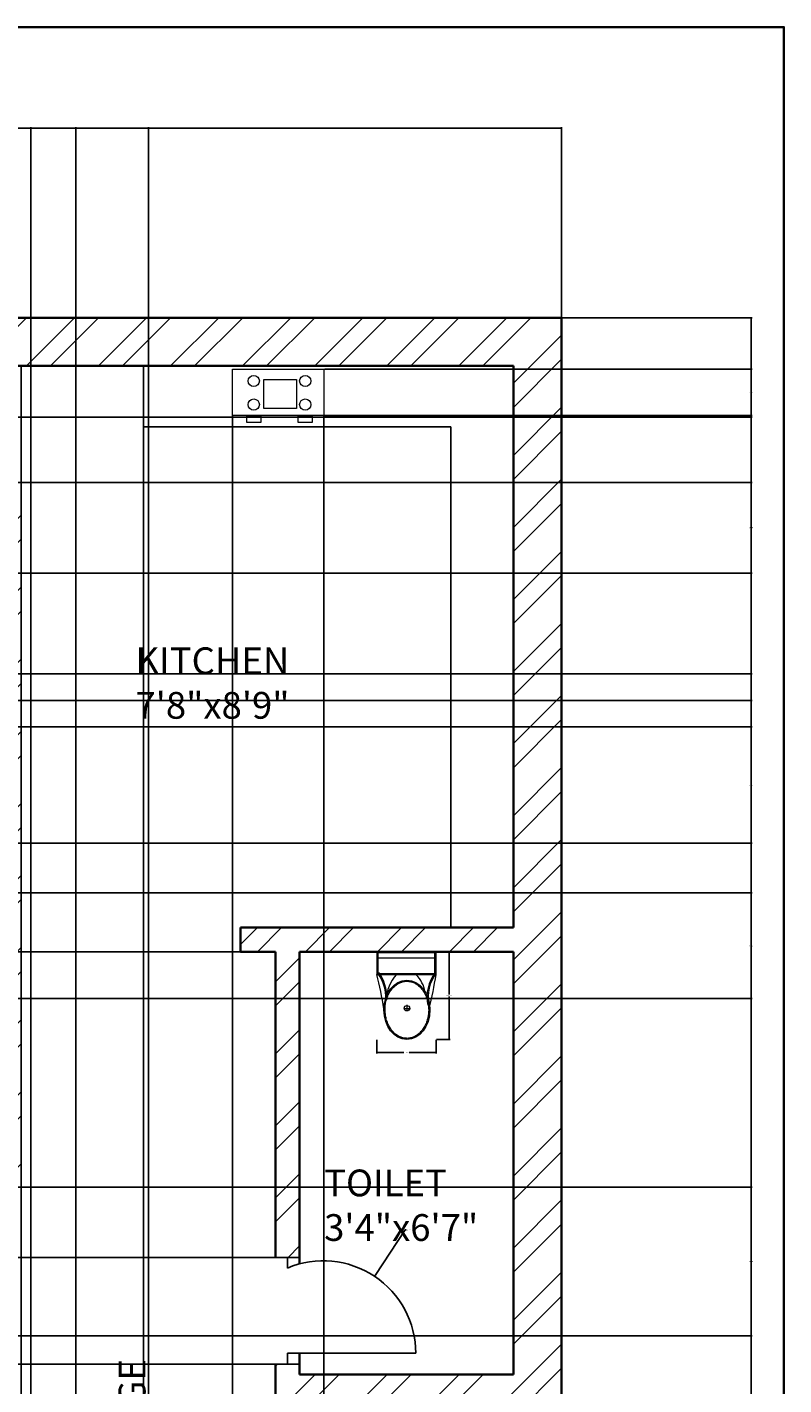
# Model space of a CAD drawing. Units: inches. Extents: x 2529 to 3014, y 1203 to 2262.
# Tile 13 of 13: x 2872 to 3014, y 2008 to 2262. Entities that reach past the tile are written whole.
import ezdxf

# ---------------------------------------------------------------- set-up
doc = ezdxf.new("R2010")
doc.units = ezdxf.units.IN
for name, color, linetype, lineweight in [('A-ANNO-DIMS', 2, 'Continuous', 18), ('A-ANNO-TTLB', 7, 'Continuous', 35), ('A-AREA-IDEN', 7, 'Continuous', 18), ('A-DOOR', 21, 'Continuous', 25), ('A-EQPM', 8, 'Continuous', 18), ('A-FLOR-CASE', 7, 'Continuous', 25), ('A-FLOR-FIXT', 8, 'Continuous', 18), ('A-WALL', 7, 'Continuous', 35), ('A-WALL-PATT', 143, 'Continuous', 13)]:
    doc.layers.add(name, color=color, linetype=linetype, lineweight=lineweight)
doc.styles.get("Standard").update_dxf_attribs({"font": 'arial.ttf'})
doc.dimstyles.get("Standard").update_dxf_attribs({"dimtxt": 0.18, "dimasz": 0.18, "dimexe": 0.18, "dimexo": 0.0625, "dimgap": 0.09, "dimtad": 0, "dimtih": 1, "dimtoh": 1, "dimdec": 4, "dimzin": 0, "dimdsep": 46, "dimtxsty": 'Standard', "dimcen": 0.09, "dimadec": 0, "dimazin": 0, "dimtfac": 1, "dimtdec": 4, "dimtofl": 0, "dimtmove": 0, "dimatfit": 3, "dimfxl": 1, "dimtolj": 1, "dimtzin": 0, "dimarcsym": 0})

# ---------------------------------------------------------------- blocks, each defined once
blk = doc.blocks.new('A$C31115884')
for p, q in [((283, 498), (223, 498)), ((258, 466), (258, 523)), ((0, 200), (0, 0)), ((520, 200), (0, 200)), ((10, 190), (10, 10)), ((510, 190), (10, 190)), ((510, 10), (510, 190)), ((520, 0), (520, 200)), ((510, 54), (0, 54)), ((10, 10), (510, 10)), ((0, 0), (520, 0))]:
    blk.add_line(p, q)
blk.add_circle((256, 496), 23.6)
for centre, radius, start, end in [((2778, -205), 2807, 165.4549, 171.7133), ((3237, 905), 2807, 188.2867, 194.5451), ((-295, 403), 365, 324.2091, 9.3499), ((-295, 403), 375, 324.2091, 9.3499), ((139, 406), 293, 315.8436, 2.6563), ((806, 403), 375, 179.2036, 215.7909), ((806, 403), 365, 170.6501, 215.7909), ((384, 406), 293, 190.2774, 224.1564)]:
    blk.add_arc(centre, radius, start, end)
blk.add_ellipse((256, 510), major_axis=(0, -261), ratio=0.772727)
blk.add_open_spline([(256, 259), (263, 259), (270, 260), (288, 262), (299, 265), (320, 273), (330, 278), (350, 291), (360, 299), (378, 316), (386, 326), (402, 347), (409, 358), (421, 383), (427, 395), (436, 422), (440, 436), (445, 465), (447, 480), (448, 509), (448, 524), (445, 553), (443, 568), (436, 596), (432, 610), (422, 636), (416, 649), (402, 672), (395, 683), (379, 703), (370, 712), (351, 728), (341, 735), (321, 746), (310, 751), (289, 757), (278, 759), (256, 761), (245, 761), (223, 757), (212, 754), (191, 746), (181, 741), (161, 728), (151, 720), (133, 703), (125, 693), (110, 672), (103, 660), (90, 636), (85, 623), (76, 596), (72, 582), (67, 553), (66, 538), (64, 509), (65, 494), (68, 465), (70, 450), (77, 422), (81, 408), (91, 382), (97, 370), (111, 346), (118, 335), (135, 316), (144, 307), (162, 291), (172, 284), (193, 273), (203, 269), (225, 262), (236, 260), (250, 259), (253, 259), (256, 259)], degree=3, knots=[0, 0, 0, 0, 0.110105, 0.110105, 0.285049, 0.285049, 0.459994, 0.459994, 0.634938, 0.634938, 0.809882, 0.809882, 0.984827, 0.984827, 1.159771, 1.159771, 1.334715, 1.334715, 1.50966, 1.50966, 1.684604, 1.684604, 1.859549, 1.859549, 2.034493, 2.034493, 2.209437, 2.209437, 2.384382, 2.384382, 2.559326, 2.559326, 2.73427, 2.73427, 2.909215, 2.909215, 3.084159, 3.084159, 3.259103, 3.259103, 3.434048, 3.434048, 3.608992, 3.608992, 3.783936, 3.783936, 3.958881, 3.958881, 4.133825, 4.133825, 4.30877, 4.30877, 4.483714, 4.483714, 4.658658, 4.658658, 4.833603, 4.833603, 5.008547, 5.008547, 5.183491, 5.183491, 5.358436, 5.358436, 5.53338, 5.53338, 5.708324, 5.708324, 5.883269, 5.883269, 6.058213, 6.058213, 6.233158, 6.233158, 6.283185, 6.283185, 6.283185, 6.283185])
blk = doc.blocks.new('*D8')
at = {"layer": 'A-ANNO-DIMS', "color": 0, "lineweight": -2, "transparency": 16777216}
for p, q in [((2948.65, 2089), (2951.23, 2089)), ((2951.05, 2088.82), (2951.05, 2080.99)), ((2951.05, 2072.78), (2951.05, 2080.62)), ((2948.65, 2072.6), (2951.23, 2072.6))]:
    blk.add_line(p, q, dxfattribs=at)
at = {"layer": 'A-ANNO-DIMS', "color": 0, "transparency": 16777216}
for points in [[(2951.02, 2088.82), (2951.08, 2088.82), (2951.05, 2089)], [(2951.02, 2072.78), (2951.08, 2072.78), (2951.05, 2072.6)]]:
    blk.add_solid(points, dxfattribs=at)
at = {"layer": 'Defpoints', "color": 0, "transparency": 16777216}
for p in [(2948.59, 2089), (2948.59, 2072.6), (2951.05, 2072.6)]:
    blk.add_point(p, dxfattribs=at)
at = {"layer": 'A-ANNO-DIMS', "color": 0, "transparency": 16777216, "insert": (2951.05, 2080.8), "char_height": 0.18, "attachment_point": 5}
blk.add_mtext('\\A1;WC 16 TYP.', dxfattribs=at)
blk = doc.blocks.new('*D9')
at = {"layer": 'A-ANNO-DIMS', "color": 0, "lineweight": -2, "transparency": 16777216}
for p, q in [((2937.52, 2072.54), (2937.52, 2069.96)), ((2948.59, 2072.54), (2948.59, 2069.96)), ((2937.7, 2070.14), (2942.54, 2070.14)), ((2948.41, 2070.14), (2943.57, 2070.14))]:
    blk.add_line(p, q, dxfattribs=at)
at = {"layer": 'A-ANNO-DIMS', "color": 0, "transparency": 16777216}
for points in [[(2937.7, 2070.17), (2937.7, 2070.11), (2937.52, 2070.14)], [(2948.41, 2070.17), (2948.41, 2070.11), (2948.59, 2070.14)]]:
    blk.add_solid(points, dxfattribs=at)
at = {"layer": 'Defpoints', "color": 0, "transparency": 16777216}
for p in [(2937.52, 2072.6), (2948.59, 2072.6), (2937.52, 2070.14)]:
    blk.add_point(p, dxfattribs=at)
at = {"layer": 'A-ANNO-DIMS', "color": 0, "transparency": 16777216, "insert": (2943.06, 2070.14), "char_height": 0.18, "attachment_point": 5}
blk.add_mtext('\\A1;11 TYP.', dxfattribs=at)
blk = doc.blocks.new('*D16')
at = {"layer": 'A-ANNO-DIMS', "color": 0, "lineweight": -2, "transparency": 16777216}
for p, q in [((2577.06, 2207.57), (2577.06, 2243.11)), ((2577.24, 2242.93), (2774.27, 2242.93)), ((2971.88, 2242.93), (2774.84, 2242.93)), ((2972.06, 2207.57), (2972.06, 2243.11))]:
    blk.add_line(p, q, dxfattribs=at)
at = {"layer": 'A-ANNO-DIMS', "color": 0, "transparency": 16777216}
for points in [[(2577.24, 2242.96), (2577.24, 2242.9), (2577.06, 2242.93)], [(2971.88, 2242.96), (2971.88, 2242.9), (2972.06, 2242.93)]]:
    blk.add_solid(points, dxfattribs=at)
at = {"layer": 'Defpoints', "color": 0, "transparency": 16777216}
for p in [(2972.06, 2242.93), (2577.06, 2207.5), (2972.06, 2207.5)]:
    blk.add_point(p, dxfattribs=at)
at = {"layer": 'A-ANNO-DIMS', "color": 0, "transparency": 16777216, "insert": (2774.56, 2242.93), "char_height": 0.18, "attachment_point": 5}
blk.add_mtext('\\A1;395', dxfattribs=at)
blk = doc.blocks.new('*D17')
at = {"layer": 'A-ANNO-DIMS', "color": 0, "lineweight": -2, "transparency": 16777216}
for p, q in [((2972.12, 2207.5), (3007.66, 2207.5)), ((3007.48, 2207.32), (3007.48, 1890.69)), ((3007.48, 1573.68), (3007.48, 1890.32)), ((2972.12, 1573.5), (3007.66, 1573.5))]:
    blk.add_line(p, q, dxfattribs=at)
at = {"layer": 'A-ANNO-DIMS', "color": 0, "transparency": 16777216}
for points in [[(3007.45, 2207.32), (3007.51, 2207.32), (3007.48, 2207.5)], [(3007.45, 1573.68), (3007.51, 1573.68), (3007.48, 1573.5)]]:
    blk.add_solid(points, dxfattribs=at)
at = {"layer": 'Defpoints', "color": 0, "transparency": 16777216}
for p in [(2972.06, 2207.5), (3007.48, 2207.5), (2972.06, 1573.5)]:
    blk.add_point(p, dxfattribs=at)
at = {"layer": 'A-ANNO-DIMS', "color": 0, "transparency": 16777216, "insert": (3007.48, 1890.5), "char_height": 0.18, "attachment_point": 5}
blk.add_mtext('\\A1;634', dxfattribs=at)
blk = doc.blocks.new('*D39')
at = {"layer": 'A-ANNO-DIMS', "color": 0, "lineweight": -2, "transparency": 16777216}
for p, q in [((2848.27, 1734.07), (2848.27, 2243.11)), ((2848.45, 2242.93), (2864.3, 2242.93)), ((2881.08, 2242.93), (2865.23, 2242.93)), ((2881.26, 1734.07), (2881.26, 2243.11))]:
    blk.add_line(p, q, dxfattribs=at)
at = {"layer": 'A-ANNO-DIMS', "color": 0, "transparency": 16777216}
for points in [[(2848.45, 2242.96), (2848.45, 2242.9), (2848.27, 2242.93)], [(2881.08, 2242.96), (2881.08, 2242.9), (2881.26, 2242.93)]]:
    blk.add_solid(points, dxfattribs=at)
at = {"layer": 'Defpoints', "color": 0, "transparency": 16777216}
for p in [(2881.26, 2242.93), (2848.27, 1734), (2881.26, 1734)]:
    blk.add_point(p, dxfattribs=at)
at = {"layer": 'A-ANNO-DIMS', "color": 0, "transparency": 16777216, "insert": (2864.76, 2242.93), "char_height": 0.18, "attachment_point": 5}
blk.add_mtext('\\A1;32.994', dxfattribs=at)
blk = doc.blocks.new('*D46')
at = {"layer": 'A-ANNO-DIMS', "color": 0, "lineweight": -2, "transparency": 16777216}
for p, q in [((2613.12, 2188.94), (3007.66, 2188.94)), ((3007.48, 2188.76), (3007.48, 2165.12)), ((3007.48, 2141.12), (3007.48, 2164.75)), ((2613.12, 2140.94), (3007.66, 2140.94))]:
    blk.add_line(p, q, dxfattribs=at)
at = {"layer": 'A-ANNO-DIMS', "color": 0, "transparency": 16777216}
for points in [[(3007.45, 2188.76), (3007.51, 2188.76), (3007.48, 2188.94)], [(3007.45, 2141.12), (3007.51, 2141.12), (3007.48, 2140.94)]]:
    blk.add_solid(points, dxfattribs=at)
at = {"layer": 'Defpoints', "color": 0, "transparency": 16777216}
for p in [(2613.06, 2188.94), (3007.48, 2188.94), (2613.06, 2140.94)]:
    blk.add_point(p, dxfattribs=at)
at = {"layer": 'A-ANNO-DIMS', "color": 0, "transparency": 16777216, "insert": (3007.48, 2164.94), "char_height": 0.18, "attachment_point": 5}
blk.add_mtext('\\A1;48', dxfattribs=at)
blk = doc.blocks.new('*D47')
at = {"layer": 'A-ANNO-DIMS', "color": 0, "lineweight": -2, "transparency": 16777216}
for p, q in [((2622.12, 2131.02), (3007.66, 2131.02)), ((3007.48, 2130.84), (3007.48, 2120.34)), ((3007.48, 2109.48), (3007.48, 2119.98)), ((2622.12, 2109.3), (3007.66, 2109.3))]:
    blk.add_line(p, q, dxfattribs=at)
at = {"layer": 'A-ANNO-DIMS', "color": 0, "transparency": 16777216}
for points in [[(3007.45, 2130.84), (3007.51, 2130.84), (3007.48, 2131.02)], [(3007.45, 2109.48), (3007.51, 2109.48), (3007.48, 2109.3)]]:
    blk.add_solid(points, dxfattribs=at)
at = {"layer": 'Defpoints', "color": 0, "transparency": 16777216}
for p in [(2622.06, 2131.02), (3007.48, 2131.02), (2622.06, 2109.3)]:
    blk.add_point(p, dxfattribs=at)
at = {"layer": 'A-ANNO-DIMS', "color": 0, "transparency": 16777216, "insert": (3007.48, 2120.16), "char_height": 0.18, "attachment_point": 5}
blk.add_mtext('\\A1;21.72', dxfattribs=at)
blk = doc.blocks.new('*D48')
at = {"layer": 'A-ANNO-DIMS', "color": 0, "lineweight": -2, "transparency": 16777216}
for p, q in [((2686.62, 2099.98), (3007.66, 2099.98)), ((3007.48, 2099.8), (3007.48, 2090.29)), ((3007.48, 2080.41), (3007.48, 2089.93)), ((2686.62, 2080.23), (3007.66, 2080.23))]:
    blk.add_line(p, q, dxfattribs=at)
at = {"layer": 'A-ANNO-DIMS', "color": 0, "transparency": 16777216}
for points in [[(3007.45, 2099.8), (3007.51, 2099.8), (3007.48, 2099.98)], [(3007.45, 2080.41), (3007.51, 2080.41), (3007.48, 2080.23)]]:
    blk.add_solid(points, dxfattribs=at)
at = {"layer": 'Defpoints', "color": 0, "transparency": 16777216}
for p in [(2686.56, 2099.98), (3007.48, 2099.98), (2686.56, 2080.23)]:
    blk.add_point(p, dxfattribs=at)
at = {"layer": 'A-ANNO-DIMS', "color": 0, "transparency": 16777216, "insert": (3007.48, 2090.11), "char_height": 0.18, "attachment_point": 5}
blk.add_mtext('\\A1;19.75', dxfattribs=at)
blk = doc.blocks.new('*D50')
at = {"layer": 'A-ANNO-DIMS', "color": 0, "lineweight": -2, "transparency": 16777216}
for p, q in [((2866.62, 2045.02), (3007.66, 2045.02)), ((3007.48, 2044.84), (3007.48, 2031.3)), ((3007.48, 2017.39), (3007.48, 2030.93)), ((2866.62, 2017.21), (3007.66, 2017.21))]:
    blk.add_line(p, q, dxfattribs=at)
at = {"layer": 'A-ANNO-DIMS', "color": 0, "transparency": 16777216}
for points in [[(3007.45, 2044.84), (3007.51, 2044.84), (3007.48, 2045.02)], [(3007.45, 2017.39), (3007.51, 2017.39), (3007.48, 2017.21)]]:
    blk.add_solid(points, dxfattribs=at)
at = {"layer": 'Defpoints', "color": 0, "transparency": 16777216}
for p in [(2866.56, 2045.02), (3007.48, 2045.02), (2866.56, 2017.21)]:
    blk.add_point(p, dxfattribs=at)
at = {"layer": 'A-ANNO-DIMS', "color": 0, "transparency": 16777216, "insert": (3007.48, 2031.12), "char_height": 0.18, "attachment_point": 5}
blk.add_mtext('\\A1;27.814', dxfattribs=at)
blk = doc.blocks.new('*D57')
at = {"layer": 'A-ANNO-DIMS', "color": 0, "lineweight": -2, "transparency": 16777216}
for p, q in [((2871.06, 2198.44), (2871.06, 1483.77)), ((2893.92, 2198.44), (2893.92, 1483.77)), ((2871.24, 1483.95), (2882.02, 1483.95)), ((2893.74, 1483.95), (2882.95, 1483.95))]:
    blk.add_line(p, q, dxfattribs=at)
at = {"layer": 'A-ANNO-DIMS', "color": 0, "transparency": 16777216}
for points in [[(2871.24, 1483.98), (2871.24, 1483.92), (2871.06, 1483.95)], [(2893.74, 1483.98), (2893.74, 1483.92), (2893.92, 1483.95)]]:
    blk.add_solid(points, dxfattribs=at)
at = {"layer": 'Defpoints', "color": 0, "transparency": 16777216}
for p in [(2871.06, 2198.5), (2893.92, 2198.5), (2893.92, 1483.95)]:
    blk.add_point(p, dxfattribs=at)
at = {"layer": 'A-ANNO-DIMS', "color": 0, "transparency": 16777216, "insert": (2882.49, 1483.95), "char_height": 0.18, "attachment_point": 5}
blk.add_mtext('\\A1;22.866', dxfattribs=at)
blk = doc.blocks.new('*D58')
at = {"layer": 'A-ANNO-DIMS', "color": 0, "lineweight": -2, "transparency": 16777216}
for p, q in [((2918.49, 2089), (2541.45, 2089)), ((2541.63, 2088.82), (2541.63, 2060.62)), ((2541.63, 2032.05), (2541.63, 2060.26)), ((2918.49, 2031.87), (2541.45, 2031.87))]:
    blk.add_line(p, q, dxfattribs=at)
at = {"layer": 'A-ANNO-DIMS', "color": 0, "transparency": 16777216}
for points in [[(2541.6, 2088.82), (2541.66, 2088.82), (2541.63, 2089)], [(2541.6, 2032.05), (2541.66, 2032.05), (2541.63, 2031.87)]]:
    blk.add_solid(points, dxfattribs=at)
at = {"layer": 'Defpoints', "color": 0, "transparency": 16777216}
for p in [(2918.56, 2089), (2541.63, 2031.87), (2918.56, 2031.87)]:
    blk.add_point(p, dxfattribs=at)
at = {"layer": 'A-ANNO-DIMS', "color": 0, "transparency": 16777216, "insert": (2541.63, 2060.44), "char_height": 0.18, "attachment_point": 5}
blk.add_mtext('\\A1;57.13', dxfattribs=at)
blk = doc.blocks.new('*D59')
at = {"layer": 'A-ANNO-DIMS', "color": 0, "lineweight": -2, "transparency": 16777216}
for p, q in [((2918.49, 2031.87), (2541.45, 2031.87)), ((2541.63, 2031.69), (2541.63, 2022.09)), ((2541.63, 2012.12), (2541.63, 2021.73)), ((2918.49, 2011.94), (2541.45, 2011.94))]:
    blk.add_line(p, q, dxfattribs=at)
at = {"layer": 'A-ANNO-DIMS', "color": 0, "transparency": 16777216}
for points in [[(2541.6, 2031.69), (2541.66, 2031.69), (2541.63, 2031.87)], [(2541.6, 2012.12), (2541.66, 2012.12), (2541.63, 2011.94)]]:
    blk.add_solid(points, dxfattribs=at)
at = {"layer": 'Defpoints', "color": 0, "transparency": 16777216}
for p in [(2918.56, 2031.87), (2541.63, 2011.94), (2918.56, 2011.94)]:
    blk.add_point(p, dxfattribs=at)
at = {"layer": 'A-ANNO-DIMS', "color": 0, "transparency": 16777216, "insert": (2541.63, 2021.91), "char_height": 0.18, "attachment_point": 5}
blk.add_mtext('\\A1;19.933', dxfattribs=at)
blk = doc.blocks.new('*D64')
at = {"layer": 'A-ANNO-DIMS', "color": 0, "lineweight": -2, "transparency": 16777216}
for p, q in [((2872.87, 1791.07), (2872.87, 2243.11)), ((2873.05, 2242.93), (2883.47, 2242.93)), ((2894.68, 2242.93), (2884.26, 2242.93)), ((2894.86, 1791.07), (2894.86, 2243.11))]:
    blk.add_line(p, q, dxfattribs=at)
at = {"layer": 'A-ANNO-DIMS', "color": 0, "transparency": 16777216}
for points in [[(2873.05, 2242.96), (2873.05, 2242.9), (2872.87, 2242.93)], [(2894.68, 2242.96), (2894.68, 2242.9), (2894.86, 2242.93)]]:
    blk.add_solid(points, dxfattribs=at)
at = {"layer": 'Defpoints', "color": 0, "transparency": 16777216}
for p in [(2894.86, 2242.93), (2872.87, 1791), (2894.86, 1791)]:
    blk.add_point(p, dxfattribs=at)
at = {"layer": 'A-ANNO-DIMS', "color": 0, "transparency": 16777216, "insert": (2883.87, 2242.93), "char_height": 0.18, "attachment_point": 5}
blk.add_mtext('\\A1;21.99', dxfattribs=at)
blk = doc.blocks.new('*D72')
at = {"layer": 'A-ANNO-DIMS', "color": 0, "lineweight": -2, "transparency": 16777216}
for p, q in [((2631.64, 2176.7), (3007.66, 2176.7)), ((3007.48, 2176.52), (3007.48, 2168.41)), ((3007.48, 2159.93), (3007.48, 2168.04)), ((2631.64, 2159.75), (3007.66, 2159.75))]:
    blk.add_line(p, q, dxfattribs=at)
at = {"layer": 'A-ANNO-DIMS', "color": 0, "transparency": 16777216}
for points in [[(3007.45, 2176.52), (3007.51, 2176.52), (3007.48, 2176.7)], [(3007.45, 2159.93), (3007.51, 2159.93), (3007.48, 2159.75)]]:
    blk.add_solid(points, dxfattribs=at)
at = {"layer": 'Defpoints', "color": 0, "transparency": 16777216}
for p in [(2631.58, 2176.7), (3007.48, 2176.7), (2631.58, 2159.75)]:
    blk.add_point(p, dxfattribs=at)
at = {"layer": 'A-ANNO-DIMS', "color": 0, "transparency": 16777216, "insert": (3007.48, 2168.22), "char_height": 0.18, "attachment_point": 5}
blk.add_mtext('\\A1;16.957', dxfattribs=at)
blk = doc.blocks.new('*D73')
at = {"layer": 'A-ANNO-DIMS', "color": 0, "lineweight": -2, "transparency": 16777216}
for p, q in [((2631.64, 2159.75), (3007.66, 2159.75)), ((3007.48, 2159.57), (3007.48, 2148.04)), ((3007.48, 2136.16), (3007.48, 2147.68)), ((2634.12, 2135.98), (3007.66, 2135.98))]:
    blk.add_line(p, q, dxfattribs=at)
at = {"layer": 'A-ANNO-DIMS', "color": 0, "transparency": 16777216}
for points in [[(3007.45, 2159.57), (3007.51, 2159.57), (3007.48, 2159.75)], [(3007.45, 2136.16), (3007.51, 2136.16), (3007.48, 2135.98)]]:
    blk.add_solid(points, dxfattribs=at)
at = {"layer": 'Defpoints', "color": 0, "transparency": 16777216}
for p in [(2631.58, 2159.75), (2634.06, 2135.98), (3007.48, 2135.98)]:
    blk.add_point(p, dxfattribs=at)
at = {"layer": 'A-ANNO-DIMS', "color": 0, "transparency": 16777216, "insert": (3007.48, 2147.86), "char_height": 0.18, "attachment_point": 5}
blk.add_mtext('\\A1;23.77', dxfattribs=at)
blk = doc.blocks.new('*D75')
at = {"layer": 'A-ANNO-DIMS', "color": 0, "lineweight": -2, "transparency": 16777216}
for p, q in [((2910.52, 2189.17), (2910.52, 1483.77)), ((2893.92, 2187.06), (2893.92, 1483.77)), ((2894.1, 1483.95), (2901.91, 1483.95)), ((2910.34, 1483.95), (2902.54, 1483.95))]:
    blk.add_line(p, q, dxfattribs=at)
at = {"layer": 'A-ANNO-DIMS', "color": 0, "transparency": 16777216}
for points in [[(2894.1, 1483.98), (2894.1, 1483.92), (2893.92, 1483.95)], [(2910.34, 1483.98), (2910.34, 1483.92), (2910.52, 1483.95)]]:
    blk.add_solid(points, dxfattribs=at)
at = {"layer": 'Defpoints', "color": 0, "transparency": 16777216}
for p in [(2910.52, 2189.24), (2893.92, 2187.12), (2910.52, 1483.95)]:
    blk.add_point(p, dxfattribs=at)
at = {"layer": 'A-ANNO-DIMS', "color": 0, "transparency": 16777216, "insert": (2902.22, 1483.95), "char_height": 0.18, "attachment_point": 5}
blk.add_mtext('\\A1;16.6', dxfattribs=at)
blk = doc.blocks.new('*D76')
at = {"layer": 'A-ANNO-DIMS', "color": 0, "lineweight": -2, "transparency": 16777216}
for p, q in [((2910.52, 2189.17), (2910.52, 1483.77)), ((2927.64, 2189.17), (2927.64, 1483.77)), ((2910.7, 1483.95), (2918.63, 1483.95)), ((2927.46, 1483.95), (2919.54, 1483.95))]:
    blk.add_line(p, q, dxfattribs=at)
at = {"layer": 'A-ANNO-DIMS', "color": 0, "transparency": 16777216}
for points in [[(2910.7, 1483.98), (2910.7, 1483.92), (2910.52, 1483.95)], [(2927.46, 1483.98), (2927.46, 1483.92), (2927.64, 1483.95)]]:
    blk.add_solid(points, dxfattribs=at)
at = {"layer": 'Defpoints', "color": 0, "transparency": 16777216}
for p in [(2910.52, 2189.24), (2927.64, 2189.24), (2927.64, 1483.95)]:
    blk.add_point(p, dxfattribs=at)
at = {"layer": 'A-ANNO-DIMS', "color": 0, "transparency": 16777216, "insert": (2919.08, 1483.95), "char_height": 0.18, "attachment_point": 5}
blk.add_mtext('\\A1;17.123', dxfattribs=at)
blk = doc.blocks.new('*D77')
at = {"layer": 'A-ANNO-DIMS', "color": 0, "lineweight": -2, "transparency": 16777216}
for p, q in [((2927.71, 2197.87), (3007.66, 2197.87)), ((3007.48, 2197.69), (3007.48, 2193.74)), ((3007.48, 2189.42), (3007.48, 2193.37)), ((2927.71, 2189.24), (3007.66, 2189.24))]:
    blk.add_line(p, q, dxfattribs=at)
at = {"layer": 'A-ANNO-DIMS', "color": 0, "transparency": 16777216}
for points in [[(3007.45, 2197.69), (3007.51, 2197.69), (3007.48, 2197.87)], [(3007.45, 2189.42), (3007.51, 2189.42), (3007.48, 2189.24)]]:
    blk.add_solid(points, dxfattribs=at)
at = {"layer": 'Defpoints', "color": 0, "transparency": 16777216}
for p in [(2927.64, 2197.87), (3007.48, 2197.87), (2927.64, 2189.24)]:
    blk.add_point(p, dxfattribs=at)
at = {"layer": 'A-ANNO-DIMS', "color": 0, "transparency": 16777216, "insert": (3007.48, 2193.55), "char_height": 0.18, "attachment_point": 5}
blk.add_mtext('\\A1;8.635', dxfattribs=at)
blk = doc.blocks.new('*D92')
at = {"layer": 'A-ANNO-DIMS', "color": 0, "lineweight": -2, "transparency": 16777216}
for p, q in [((2942.82, 2036.99), (2937.18, 2028.5)), ((2943, 2036.99), (2942.82, 2036.99)), ((2927.43, 2013.94), (2927.61, 2013.94)), ((2927.52, 2013.85), (2927.52, 2014.03))]:
    blk.add_line(p, q, dxfattribs=at)
at = {"layer": 'A-ANNO-DIMS', "color": 0, "transparency": 16777216}
blk.add_solid([(2937.15, 2028.51), (2937.2, 2028.48), (2937.08, 2028.35)], dxfattribs=at)
at = {"layer": 'Defpoints', "color": 0, "transparency": 16777216}
for p in [(2937.08, 2028.35), (2927.52, 2013.94)]:
    blk.add_point(p, dxfattribs=at)
at = {"layer": 'A-ANNO-DIMS', "color": 0, "transparency": 16777216, "insert": (2943.48, 2036.99), "char_height": 0.18, "attachment_point": 5}
blk.add_mtext('\\A1;R17.29', dxfattribs=at)

msp = doc.modelspace()

# ---------------------------------------------------------------- hatches: boundary and pattern name
at = {"layer": 'A-WALL-PATT'}
h = msp.add_hatch(dxfattribs=at)
h.set_pattern_fill('ANSI32', color=256)
h.paths.add_polyline_path([(2686.5554, 2106.5032), (2622.0554, 2106.5032), (2622.0554, 2109.2964), (2617.4223, 2109.2964), (2613.0554, 2109.2964), (2613.0554, 2106.5032), (2577.0554, 2106.5032), (2577.0554, 2092.6918), (2586.0554, 2092.6918), (2586.0554, 2102.0032), (2682.0554, 2102.0032), (2682.0554, 2099.9833), (2686.5554, 2099.9833), (2686.5554, 2102.0032)])
h.paths.add_polyline_path([(2695.2249, 2054.0032), (2686.5554, 2054.0032), (2686.5554, 2080.2316), (2684.3054, 2080.2316), (2682.0554, 2080.2316), (2682.0554, 2054.0032), (2586.0554, 2054.0032), (2586.0554, 2068.6918), (2577.0554, 2068.6918), (2577.0554, 2019.1229), (2586.0554, 2019.1229), (2586.0554, 2049.5032), (2695.2249, 2049.5032)])
h.paths.add_polyline_path([(2737.5554, 2049.5032), (2866.5554, 2049.5032), (2866.5554, 2045.0233), (2871.0554, 2045.0233), (2871.0554, 2049.5032), (2871.0554, 2172.5032), (2866.5554, 2172.5032), (2829.1265, 2172.5032), (2829.1265, 2168.0032), (2866.5554, 2168.0032), (2866.5554, 2054.0032), (2737.5554, 2054.0032), (2737.5554, 2056.4892), (2735.3054, 2056.4892), (2733.0554, 2056.4892), (2733.0554, 2049.5032), (2733.0554, 1917.5032), (2733.0554, 1913.0032), (2871.0554, 1913.0032), (2871.0554, 1924.9149), (2868.8054, 1924.9149), (2866.5554, 1924.9149), (2866.5554, 1917.5032), (2737.5554, 1917.5032)], flags=17)
h.paths.add_polyline_path([(2972.0554, 2207.5032), (2613.0554, 2207.5032), (2613.0554, 2205.5032), (2613.0554, 2188.9366), (2622.0554, 2188.9366), (2622.0554, 2198.5032), (2733.0554, 2198.5032), (2733.0554, 2084.8053), (2735.3054, 2084.8053), (2737.5554, 2084.8053), (2737.5554, 2168.0032), (2769.1265, 2168.0032), (2769.1265, 2170.2532), (2769.1265, 2172.5032), (2737.5554, 2172.5032), (2737.5554, 2198.5032), (2963.0554, 2198.5032), (2963.0554, 2093.5032), (2912.0586, 2093.5032), (2912.0586, 2089.0032), (2918.5554, 2089.0032), (2918.5554, 2031.8749), (2923.0554, 2031.8749), (2923.0554, 2089.0032), (2963.0554, 2089.0032), (2963.0554, 2010.0032), (2923.0554, 2010.0032), (2923.0554, 2011.9417), (2918.5554, 2011.9417), (2918.5554, 2003.1338), (2923.0554, 2003.1338), (2923.0554, 2005.5032), (2963.0554, 2005.5032), (2963.0554, 1917.5032), (2963.0554, 1691.0776), (2972.0554, 1691.0776), (2972.0554, 1917.5032)])
h.paths.add_polyline_path([(2963.0554, 1945.5032), (2923.0554, 1945.5032), (2923.0554, 1983.0571), (2920.8054, 1983.0571), (2918.5554, 1983.0571), (2918.5554, 1941.0032), (2963.0554, 1941.0032)], flags=17)
h.paths.add_polyline_path([(2930.3679, 1788.7532), (2930.3679, 1791.0032), (2894.8637, 1791.0032), (2894.8637, 1786.5032), (2900.5554, 1786.5032), (2900.5554, 1784.6931), (2905.0554, 1784.6931), (2905.0554, 1786.5032), (2930.3679, 1786.5032)], flags=17)
h.paths.add_polyline_path([(2963.0554, 1791.0032), (2954.3679, 1791.0032), (2954.3679, 1786.5032), (2963.0554, 1786.5032)], flags=17)
h.paths.add_polyline_path([(2871.0554, 1853.0032), (2919.0554, 1853.0032), (2919.0554, 1847.0972), (2923.5554, 1847.0972), (2923.5554, 1853.0032), (2923.5554, 1857.5032), (2871.0554, 1857.5032), (2871.0554, 1871.7024), (2866.5554, 1871.7024), (2866.5554, 1791.0032), (2737.5554, 1791.0032), (2737.5554, 1806.6712), (2735.3054, 1806.6712), (2733.0554, 1806.6712), (2733.0554, 1791.0032), (2733.0554, 1786.5032), (2733.0554, 1780.6235), (2737.5554, 1780.6235), (2737.5554, 1786.5032), (2872.8745, 1786.5032), (2872.8745, 1788.7532), (2872.8745, 1791.0032), (2871.0554, 1791.0032)], flags=17)
h.paths.add_polyline_path([(2844.0554, 1734.0032), (2848.2652, 1734.0032), (2848.2652, 1738.5032), (2800.0167, 1738.5032), (2800.0167, 1734.0032), (2839.5554, 1734.0032), (2839.5554, 1582.5032), (2792.3334, 1582.5032), (2792.3334, 1573.5032), (2871.4433, 1573.5032), (2871.4433, 1578.0032), (2871.4433, 1582.5032), (2844.0554, 1582.5032)])
h.paths.add_polyline_path([(2972.0554, 1631.0776), (2963.0554, 1631.0776), (2963.0554, 1582.5032), (2931.4433, 1582.5032), (2931.4433, 1573.5032), (2972.0554, 1573.5032)])
h.paths.add_polyline_path([(2756.3334, 1582.5032), (2737.5554, 1582.5032), (2737.5554, 1734.0032), (2744.3201, 1734.0032), (2744.3201, 1738.5032), (2737.5554, 1738.5032), (2737.5554, 1746.0094), (2733.0554, 1746.0094), (2733.0554, 1738.5032), (2733.0554, 1612.5032), (2728.2475, 1612.5032), (2728.2475, 1603.5032), (2733.0554, 1603.5032), (2733.0554, 1582.5032), (2733.0554, 1573.5032), (2756.3334, 1573.5032), (2756.3334, 1578.0032)])
h.paths.add_polyline_path([(2695.7662, 1612.5032), (2658.4771, 1612.5032), (2658.4771, 1603.5032), (2695.7662, 1603.5032), (2695.7662, 1608.0032)])
h.paths.add_polyline_path([(2586.0554, 1686.9483), (2577.0554, 1686.9483), (2577.0554, 1603.5032), (2598.4771, 1603.5032), (2598.4771, 1608.0032), (2598.4771, 1612.5032), (2586.0554, 1612.5032)])
h.paths.add_polyline_path([(2683.2727, 1791.0032), (2586.0554, 1791.0032), (2586.0554, 1815.6736), (2581.5554, 1815.6736), (2577.0554, 1815.6736), (2577.0554, 1746.9483), (2586.0554, 1746.9483), (2586.0554, 1786.5032), (2683.2727, 1786.5032)])
h.paths.add_polyline_path([(2586.0554, 1959.1229), (2577.0554, 1959.1229), (2577.0554, 1875.6736), (2586.0554, 1875.6736), (2586.0554, 1913.0032), (2683.2727, 1913.0032), (2683.2727, 1917.5032), (2586.0554, 1917.5032)])

# ---------------------------------------------------------------- linework, layer by layer
at = {"layer": 'A-ANNO-TTLB'}
msp.add_lwpolyline([(2528.6765, 2261.8165), (3013.6003, 2261.8165), (3013.6003, 1455.1523), (2528.6765, 1455.1523)], close=True, dxfattribs=at)
at = {"layer": 'A-DOOR'}
for p, q in [((2918.5554, 2031.8749), (2923.0554, 2031.8749)), ((2923.0554, 2031.8749), (2920.8054, 2031.8749)), ((2920.8054, 2031.8749), (2920.8054, 2029.8749)), ((2920.8054, 2011.9417), (2920.8054, 2013.9417)), ((2920.8054, 2013.9417), (2944.8054, 2013.9417)), ((2923.0554, 2011.9417), (2918.5554, 2011.9417)), ((2918.5554, 2011.9417), (2920.8054, 2011.9417))]:
    msp.add_line(p, q, dxfattribs=at)
msp.add_arc((2927.5164, 2013.9417), 17.2889, 0, 112.840809, dxfattribs=at)
at = {"layer": 'A-EQPM'}
for points in [[(2910.5203, 2197.8718), (2927.6434, 2197.8718), (2927.6434, 2189.237), (2910.5203, 2189.237)], [(2916.4015, 2195.9611), (2922.5335, 2195.9611), (2922.5335, 2190.5448), (2916.4015, 2190.5448)], [(2913.2089, 2189.237), (2915.8212, 2189.237), (2915.8212, 2187.9409), (2913.2089, 2187.9409)], [(2922.8192, 2189.237), (2925.4315, 2189.237), (2925.4315, 2187.9409), (2922.8192, 2187.9409)]]:
    msp.add_lwpolyline(points, close=True, dxfattribs=at)
for centre in [(2914.5246, 2195.6798), (2924.1349, 2195.6798), (2914.5246, 2191.2766), (2924.1349, 2191.2766)]:
    msp.add_circle(centre, 1.0484, dxfattribs=at)
at = {"layer": 'A-FLOR-CASE'}
for p, q in [((2893.9216, 2198.5032), (2893.9216, 2187.1225)), ((2893.9216, 2187.1225), (2951.356, 2187.1225)), ((2951.356, 2187.1225), (2951.356, 2093.5032))]:
    msp.add_line(p, q, dxfattribs=at)
at = {"layer": 'A-WALL'}
for p, q in [((2613.0554, 2207.5032), (2972.0554, 2207.5032)), ((2972.0554, 2207.5032), (2972.0554, 1917.5032)), ((2737.5554, 2198.5032), (2963.0554, 2198.5032)), ((2963.0554, 2198.5032), (2963.0554, 2093.5032)), ((2963.0554, 2198.5032), (2963.0554, 2093.5032)), ((2963.0554, 2093.5032), (2912.0586, 2093.5032)), ((2912.0586, 2093.5032), (2912.0586, 2089.0032)), ((2912.0586, 2089.0032), (2918.5554, 2089.0032)), ((2918.5554, 2089.0032), (2918.5554, 2031.8749)), ((2923.0554, 2089.0032), (2923.0554, 2030.6451)), ((2923.0554, 2089.0032), (2963.0554, 2089.0032)), ((2963.0554, 2089.0032), (2963.0554, 2010.0032)), ((2923.0554, 2013.9417), (2923.0554, 2010.0032)), ((2918.5554, 2011.9417), (2918.5554, 2003.1338)), ((2923.0554, 2010.0032), (2963.0554, 2010.0032))]:
    msp.add_line(p, q, dxfattribs=at)

# ---------------------------------------------------------------- block references
at = {"layer": 'A-FLOR-FIXT', "xscale": 0.021283599635143, "yscale": 0.021283599635143, "zscale": 0.021283599635143, "rotation": 180}
msp.add_blockref('A$C31115884', (2948.5891, 2089.0032), dxfattribs=at)

# ---------------------------------------------------------------- texts
at = {"layer": 'A-AREA-IDEN', "char_height": 5, "attachment_point": 1}
for s, width, insert in [('KITCHEN \\P7\'8"x8\'9"', 148.086301, (2892.4052, 2145.891)), ('TOILET\\P3\'4"x6\'7"', 148.634096, (2927.6687, 2048.2874))]:
    msp.add_mtext_dynamic_manual_height_columns(s, width=width, gutter_width=12.5, heights=[0], dxfattribs=dict(at, insert=insert))
at = {"layer": 'A-AREA-IDEN', "insert": (2889.2755, 1950.9524), "char_height": 5, "attachment_point": 1, "rotation": 90}
msp.add_mtext_dynamic_manual_height_columns('4\'0" WIDE PASSAGE', width=108.755322, gutter_width=12.5, heights=[0], dxfattribs=at)

# ---------------------------------------------------------------- dimensions: what is measured, and where the dimension line sits
at = {"layer": 'A-ANNO-DIMS'}
for base, p1, p2, override, picture, middle in [((2972.0554, 2242.9282), (2577.0554, 2207.5032), (2972.0554, 2207.5032), {"dimdec": 0, "dimlfac": 1, "dimrnd": 0, "dimzin": 0, "dimdsep": 46, "dimlunit": 2}, '*D16', (2774.5554, 2242.9282)), ((2881.259, 2242.9282), (2848.2652, 1734.0032), (2881.259, 1734.0032), {"dimdec": 3, "dimlfac": 1, "dimrnd": 0, "dimzin": 0, "dimdsep": 46, "dimlunit": 2}, '*D39', (2864.7621, 2242.9282)), ((2894.8637, 2242.9282), (2872.8745, 1791.0032), (2894.8637, 1791.0032), {"dimdec": 2, "dimlfac": 1, "dimrnd": 0, "dimzin": 0, "dimdsep": 46, "dimlunit": 2}, '*D64', (2883.8691, 2242.9282)), ((2893.9216, 1483.9492), (2871.0554, 2198.5032), (2893.9216, 2198.5032), {"dimdec": 3, "dimlfac": 1, "dimrnd": 0, "dimzin": 0, "dimdsep": 46, "dimlunit": 2}, '*D57', (2882.4885, 1483.9492)), ((2910.5203, 1483.9492), (2893.9216, 2187.1225), (2910.5203, 2189.237), {"dimdec": 1, "dimlfac": 1, "dimrnd": 0, "dimzin": 0, "dimdsep": 46, "dimlunit": 2}, '*D75', (2902.2209, 1483.9492)), ((2927.6434, 1483.9492), (2910.5203, 2189.237), (2927.6434, 2189.237), {"dimdec": 3, "dimlfac": 1, "dimrnd": 0, "dimzin": 0, "dimdsep": 46, "dimlunit": 2}, '*D76', (2919.0819, 1483.9492))]:
    dim = msp.add_linear_dim(base=base, p1=p1, p2=p2, dimstyle='Standard', override=override, dxfattribs=at)
    dim.commit()
    dim.dimension.update_dxf_attribs({"geometry": picture, "text_midpoint": middle})
for base, p1, p2, override, picture, middle in [((3007.4804, 2207.5032), (2972.0554, 1573.5032), (2972.0554, 2207.5032), {"dimdec": 0, "dimlfac": 1, "dimrnd": 0, "dimzin": 0, "dimdsep": 46, "dimlunit": 2}, '*D17', (3007.4804, 1890.5032)), ((3007.4804, 2197.8718), (2927.6434, 2189.237), (2927.6434, 2197.8718), {"dimdec": 3, "dimlfac": 1, "dimrnd": 0, "dimzin": 0, "dimdsep": 46, "dimlunit": 2}, '*D77', (3007.4804, 2193.5544)), ((3007.4804, 2188.9366), (2613.0554, 2140.9366), (2613.0554, 2188.9366), {"dimdec": 0, "dimlfac": 1, "dimrnd": 0, "dimzin": 0, "dimdsep": 46, "dimlunit": 2}, '*D46', (3007.4804, 2164.9366)), ((3007.4804, 2176.7033), (2631.5753, 2159.7466), (2631.5753, 2176.7033), {"dimdec": 3, "dimlfac": 1, "dimrnd": 0, "dimzin": 0, "dimdsep": 46, "dimlunit": 2}, '*D72', (3007.4804, 2168.225)), ((3007.4804, 2135.9767), (2631.5753, 2159.7466), (2634.0572, 2135.9767), {"dimdec": 2, "dimlfac": 1, "dimrnd": 0, "dimzin": 0, "dimdsep": 46, "dimlunit": 2}, '*D73', (3007.4804, 2147.8617)), ((3007.4804, 2131.0168), (2622.0554, 2109.2964), (2622.0554, 2131.0168), {"dimdec": 2, "dimlfac": 1, "dimrnd": 0, "dimzin": 0, "dimdsep": 46, "dimlunit": 2}, '*D47', (3007.4804, 2120.1566)), ((3007.4804, 2099.9833), (2686.5554, 2080.2316), (2686.5554, 2099.9833), {"dimdec": 2, "dimlfac": 1, "dimrnd": 0, "dimzin": 0, "dimdsep": 46, "dimlunit": 2}, '*D48', (3007.4804, 2090.1074)), ((2541.6304, 2031.8749), (2918.5554, 2089.0032), (2918.5554, 2031.8749), {"dimdec": 2, "dimlfac": 1, "dimrnd": 0, "dimzin": 0, "dimdsep": 46, "dimlunit": 2}, '*D58', (2541.6304, 2060.4391)), ((3007.4804, 2045.0233), (2866.5554, 2017.2091), (2866.5554, 2045.0233), {"dimdec": 3, "dimlfac": 1, "dimrnd": 0, "dimzin": 0, "dimdsep": 46, "dimlunit": 2}, '*D50', (3007.4804, 2031.1162)), ((2541.6304, 2011.9417), (2918.5554, 2031.8749), (2918.5554, 2011.9417), {"dimdec": 3, "dimlfac": 1, "dimrnd": 0, "dimzin": 0, "dimdsep": 46, "dimlunit": 2}, '*D59', (2541.6304, 2021.9083))]:
    dim = msp.add_linear_dim(base=base, p1=p1, p2=p2, angle=90, dimstyle='Standard', override=override, dxfattribs=at)
    dim.commit()
    dim.dimension.update_dxf_attribs({"geometry": picture, "text_midpoint": middle})
for base, p1, p2, angle, text, picture, middle in [((2951.0492, 2072.6027), (2948.5891, 2089.0032), (2948.5891, 2072.6027), 270, 'WC <> TYP.', '*D8', (2951.0492, 2080.803)), ((2937.5216, 2070.1427), (2948.5891, 2072.6027), (2937.5216, 2072.6027), 180, '<> TYP.', '*D9', (2943.0554, 2070.1427))]:
    dim = msp.add_linear_dim(base=base, p1=p1, p2=p2, angle=angle, text=text, dimstyle='Standard', override={"dimdec": 0, "dimlfac": 1, "dimrnd": 0, "dimzin": 0, "dimdsep": 46, "dimlunit": 2}, dxfattribs=at)
    dim.commit()
    dim.dimension.update_dxf_attribs({"geometry": picture, "text_midpoint": middle})
dim = msp.add_radius_dim(center=(2927.5164, 2013.9417), mpoint=(2937.0791, 2028.3452), dimstyle='Standard', override={"dimdec": 2, "dimlfac": 1, "dimrnd": 0, "dimzin": 0, "dimdsep": 46, "dimlunit": 2}, dxfattribs=at)
dim.commit()
dim.dimension.update_dxf_attribs({"geometry": '*D92', "text_midpoint": (2943.4768, 2036.9873), "dimtype": 164})

doc.saveas('drawing.dxf')
